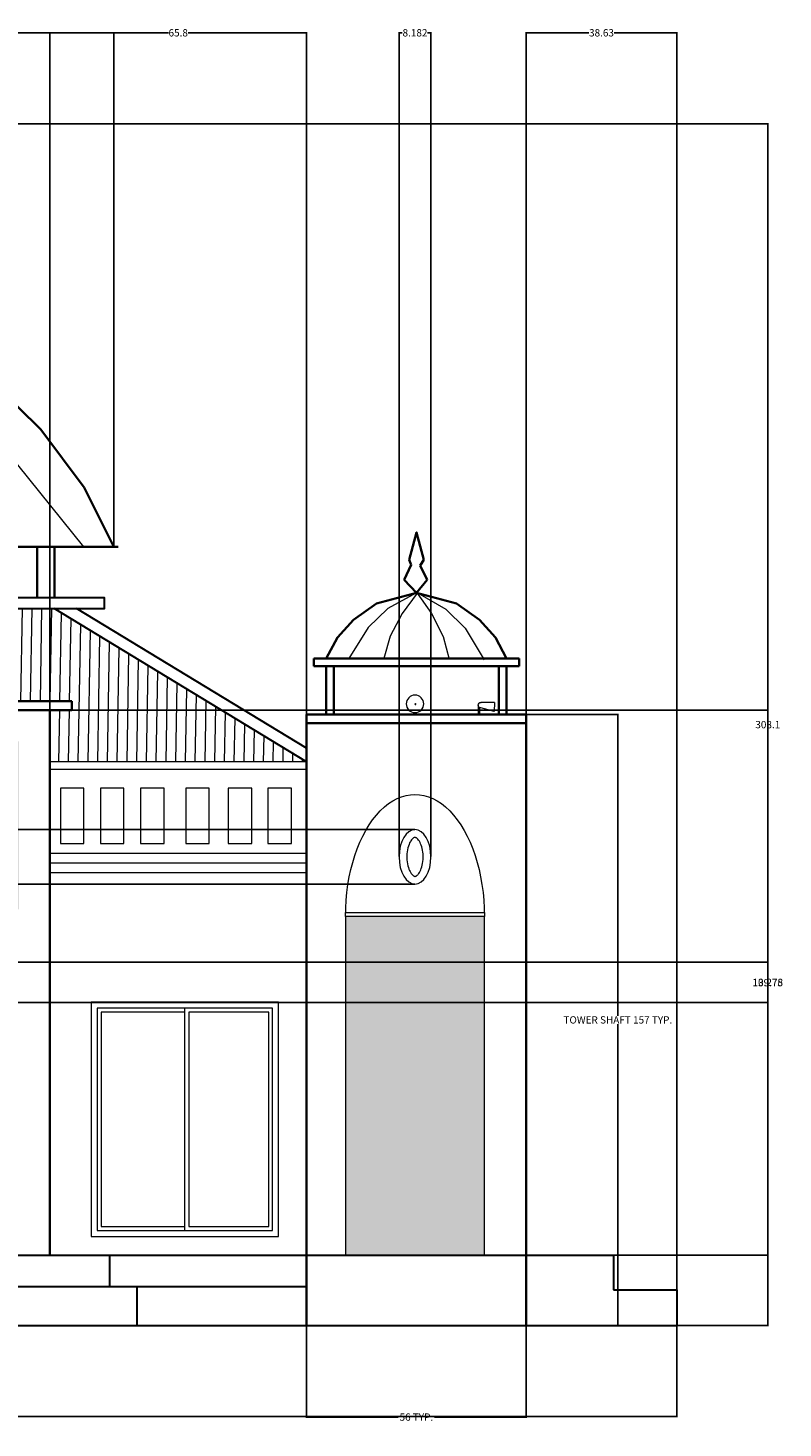
# Model space of a CAD drawing. Units: inches. Extents: x 4 to 523, y 84 to 443.
# Tile 3 of 3: x 329 to 523, y 84 to 443. Entities that reach past the tile are written whole.
import ezdxf

# ---------------------------------------------------------------- set-up
doc = ezdxf.new("R2010")
doc.units = ezdxf.units.IN
doc.header["$MEASUREMENT"] = 0
for name, color, linetype, lineweight in [('A-ANNO-DIMS', 2, 'Continuous', 18), ('A-EQPM', 8, 'Continuous', 18), ('A-FLOR-STRS', 7, 'Continuous', 30), ('A-GLAZ', 4, 'Continuous', 18), ('A-ROOF', 7, 'Continuous', 30), ('A-ROOF-DETL', 3, 'Continuous', 18), ('A-ROOF-DOME', 7, 'Continuous', 35), ('A-ROOF-PATT', 252, 'Continuous', 13), ('A-WALL', 7, 'Continuous', 35), ('A-WALL-PATT', 252, 'Continuous', 13), ('A-WALL-PORT', 7, 'Continuous', 35), ('A-WALL-TRIM', 3, 'Continuous', 18)]:
    doc.layers.add(name, color=color, linetype=linetype, lineweight=lineweight)
doc.styles.get("Standard").update_dxf_attribs({"font": 'arial.ttf'})
doc.dimstyles.get("Standard").update_dxf_attribs({"dimtxt": 1.875, "dimasz": 0.18, "dimexe": 0.18, "dimexo": 0.0625, "dimgap": 0.09, "dimtad": 0, "dimtih": 1, "dimtoh": 1, "dimdec": 4, "dimzin": 0, "dimdsep": 46, "dimlunit": 4, "dimtxsty": 'Standard', "dimcen": 0.09, "dimadec": 0, "dimazin": 0, "dimtfac": 1, "dimtdec": 4, "dimtofl": 0, "dimtmove": 0, "dimatfit": 3, "dimfxl": 1, "dimtolj": 1, "dimtzin": 0, "dimarcsym": 0})

# ---------------------------------------------------------------- blocks, each defined once
blk = doc.blocks.new('*U2')
for p, q in [((1.5, 1.5), (1.5, 58.5)), ((1.5, 58.5), (24, 58.5)), ((24, 1.5), (24, 58.5)), ((24, 58.5), (46.5, 58.5)), ((46.5, 58.5), (46.5, 1.5)), ((24, 1.5), (1.5, 1.5)), ((46.5, 1.5), (24, 1.5))]:
    blk.add_line(p, q)
blk.add_lwpolyline([(0, 0), (0, 60), (48, 60), (48, 0)], close=True)
for points in [[(23, 57.5), (23, 2.5), (2.5, 2.5), (2.5, 57.5), (23, 57.5)], [(24, 57.5), (45.5, 57.5), (45.5, 2.5), (24, 2.5)]]:
    blk.add_lwpolyline(points)
blk = doc.blocks.new('CUPOLA-PROFILE')
for p, q in [((52.59, 14.33), (0, 14.33)), ((0, 14.33), (0, 12.33)), ((0, 12.33), (52.59, 12.33)), ((3.17, 3.77), (3.17, 12.33)), ((5.17, 3.77), (5.17, 12.33)), ((47.49, 3.77), (47.49, 12.33)), ((49.49, 3.77), (49.49, 12.33)), ((52.59, 12.33), (52.59, 14.33)), ((3.17, 3.77), (3.17, 0)), ((5.17, 3.77), (5.17, 0)), ((47.49, 3.77), (47.49, 0)), ((49.49, 3.77), (49.49, 0))]:
    blk.add_line(p, q)
for points in [[(24.44, 39.59), (26.29, 46.64), (28.15, 39.59)], [(25.33, 38.18), (24.44, 39.59)], [(28.15, 39.59), (27.62, 38.34)], [(23.56, 34.47), (25.33, 38.18)], [(29.42, 34.47), (27.62, 38.34)], [(23.56, 34.47), (26.29, 31.2)], [(26.29, 31.2), (29.42, 34.47)], [(3.17, 14.33), (6, 19.75), (10.13, 24.22), (16.05, 28.42), (21.12, 29.8), (26.29, 31.2)], [(49.42, 14.33), (46.59, 19.75), (42.46, 24.22), (36.53, 28.42), (31.46, 29.8), (26.29, 31.2)]]:
    blk.add_lwpolyline(points)
blk = doc.blocks.new('TOWER-LOUDSPEAKERS')
for p, q in [((3.88, 1.79), (3.88, 0)), ((4.17, 2.36), (4.17, 0))]:
    blk.add_line(p, q)
for points in [[(0, 3.08), (0.04, 0.72), (3.47, 1.65)], [(0, 3.08), (3.47, 3.08)]]:
    blk.add_lwpolyline(points)
for centre, radius in [((20.39, 2.69), 2.24), ((20.27, 2.65), 0.127)]:
    blk.add_circle(centre, radius)
blk.add_arc((3.46, 2.36), 0.712, 271.2716, 91.2716)
blk = doc.blocks.new('TOWER-SHAFT')
for p, q in [((0, 0), (0, 156.67)), ((0, 156.67), (56.33, 156.67)), ((0, 154.45), (56.33, 154.45)), ((56.33, 156.67), (56.33, 0))]:
    blk.add_line(p, q)
blk = doc.blocks.new('NICHE-ARCH-MEDALLION')
blk.add_ellipse((17.8, 0), major_axis=(0, 31.26), ratio=0.569254, start_param=4.712389, end_param=7.853982)
blk.add_ellipse((17.8, 15.26), major_axis=(0, 6.99), ratio=0.584915)
blk.add_open_spline([(17.8, 20.25), (17.75, 20.25), (17.71, 20.25), (17.59, 20.21), (17.51, 20.17), (17.31, 20.03), (17.19, 19.93), (16.94, 19.66), (16.81, 19.49), (16.45, 18.9), (16.23, 18.42), (15.9, 17.3), (15.78, 16.67), (15.68, 15.37), (15.7, 14.7), (15.86, 13.43), (16, 12.82), (16.37, 11.77), (16.6, 11.33), (17.01, 10.76), (17.18, 10.58), (17.48, 10.36), (17.59, 10.31), (17.73, 10.26), (17.78, 10.26), (17.87, 10.27), (17.93, 10.28), (18.1, 10.35), (18.21, 10.42), (18.46, 10.64), (18.61, 10.8), (18.9, 11.2), (19.04, 11.44), (19.4, 12.22), (19.6, 12.82), (19.85, 14.13), (19.9, 14.84), (19.86, 16.25), (19.77, 16.94), (19.45, 18.19), (19.23, 18.74), (18.8, 19.48), (18.6, 19.73), (18.25, 20.07), (18.1, 20.16), (17.91, 20.24), (17.85, 20.25), (17.8, 20.25)], degree=3, knots=[0, 0, 0, 0, 0.190161, 0.190161, 0.380322, 0.380322, 0.570483, 0.570483, 0.760644, 0.760644, 1.099719, 1.099719, 1.438794, 1.438794, 1.77787, 1.77787, 2.116945, 2.116945, 2.45602, 2.45602, 2.714331, 2.714331, 2.972641, 2.972641, 3.185337, 3.185337, 3.398033, 3.398033, 3.610729, 3.610729, 3.823425, 3.823425, 4.03612, 4.03612, 4.39902, 4.39902, 4.76192, 4.76192, 5.124819, 5.124819, 5.487719, 5.487719, 5.764017, 5.764017, 6.040315, 6.040315, 6.283185, 6.283185, 6.283185, 6.283185])
blk = doc.blocks.new('FRIEZE-INSET')
blk.add_lwpolyline([(0, 14.2), (6.01, 14.2), (6.01, 0), (0, 0)], close=True)
blk = doc.blocks.new('*D9')
at = {"layer": 'A-ANNO-DIMS', "color": 0, "lineweight": -2, "transparency": 16777216}
for p, q in [((456.93, 267.13), (480.55, 267.13)), ((480.37, 266.95), (480.37, 189.86)), ((480.37, 110.64), (480.37, 187.74)), ((456.93, 110.46), (480.55, 110.46))]:
    blk.add_line(p, q, dxfattribs=at)
at = {"layer": 'A-ANNO-DIMS', "color": 0, "transparency": 16777216}
for points in [[(480.34, 266.95), (480.4, 266.95), (480.37, 267.13)], [(480.34, 110.64), (480.4, 110.64), (480.37, 110.46)]]:
    blk.add_solid(points, dxfattribs=at)
at = {"layer": 'Defpoints', "color": 0, "transparency": 16777216}
for p in [(456.87, 267.13), (480.37, 267.13), (456.87, 110.46)]:
    blk.add_point(p, dxfattribs=at)
at = {"layer": 'A-ANNO-DIMS', "color": 0, "transparency": 16777216, "insert": (480.37, 188.8), "char_height": 1.875, "attachment_point": 5}
blk.add_mtext('\\A1;TOWER SHAFT 157 TYP.', dxfattribs=at)
blk = doc.blocks.new('*D10')
at = {"layer": 'A-ANNO-DIMS', "color": 0, "lineweight": -2, "transparency": 16777216}
for p, q in [((400.53, 110.4), (400.53, 86.78)), ((456.87, 110.4), (456.87, 86.78)), ((400.71, 86.96), (424.05, 86.96)), ((456.69, 86.96), (433.35, 86.96))]:
    blk.add_line(p, q, dxfattribs=at)
at = {"layer": 'A-ANNO-DIMS', "color": 0, "transparency": 16777216}
for points in [[(400.71, 86.99), (400.71, 86.93), (400.53, 86.96)], [(456.69, 86.99), (456.69, 86.93), (456.87, 86.96)]]:
    blk.add_solid(points, dxfattribs=at)
at = {"layer": 'Defpoints', "color": 0, "transparency": 16777216}
for p in [(400.53, 110.46), (456.87, 110.46), (456.87, 86.96)]:
    blk.add_point(p, dxfattribs=at)
at = {"layer": 'A-ANNO-DIMS', "color": 0, "transparency": 16777216, "insert": (428.7, 86.96), "char_height": 1.875, "attachment_point": 5}
blk.add_mtext('\\A1;56 TYP.', dxfattribs=at)
blk = doc.blocks.new('*D19')
at = {"layer": 'A-ANNO-DIMS', "color": 0, "lineweight": -2, "transparency": 16777216}
for p, q in [((30.92, 110.4), (30.92, 86.96)), ((495.5, 110.4), (495.5, 86.96)), ((31.1, 87.14), (259.92, 87.14)), ((495.32, 87.14), (266.5, 87.14))]:
    blk.add_line(p, q, dxfattribs=at)
at = {"layer": 'A-ANNO-DIMS', "color": 0, "transparency": 16777216}
for points in [[(31.1, 87.17), (31.1, 87.11), (30.92, 87.14)], [(495.32, 87.17), (495.32, 87.11), (495.5, 87.14)]]:
    blk.add_solid(points, dxfattribs=at)
at = {"layer": 'Defpoints', "color": 0, "transparency": 16777216}
for p in [(30.92, 110.46), (495.5, 110.46), (495.5, 87.14)]:
    blk.add_point(p, dxfattribs=at)
at = {"layer": 'A-ANNO-DIMS', "color": 0, "transparency": 16777216, "insert": (263.21, 87.14), "char_height": 1.875, "attachment_point": 5}
blk.add_mtext('\\A1;464.6', dxfattribs=at)
blk = doc.blocks.new('*D20')
at = {"layer": 'A-ANNO-DIMS', "color": 0, "lineweight": -2, "transparency": 16777216}
for p, q in [((259.93, 418.56), (519, 418.56)), ((518.82, 418.38), (518.82, 265.56)), ((518.82, 110.64), (518.82, 263.46)), ((495.56, 110.46), (519, 110.46))]:
    blk.add_line(p, q, dxfattribs=at)
at = {"layer": 'A-ANNO-DIMS', "color": 0, "transparency": 16777216}
for points in [[(518.79, 418.38), (518.85, 418.38), (518.82, 418.56)], [(518.79, 110.64), (518.85, 110.64), (518.82, 110.46)]]:
    blk.add_solid(points, dxfattribs=at)
at = {"layer": 'Defpoints', "color": 0, "transparency": 16777216}
for p in [(259.87, 418.56), (518.82, 418.56), (495.5, 110.46)]:
    blk.add_point(p, dxfattribs=at)
at = {"layer": 'A-ANNO-DIMS', "color": 0, "transparency": 16777216, "insert": (518.82, 264.51), "char_height": 1.875, "attachment_point": 5}
blk.add_mtext('\\A1;308.1', dxfattribs=at)
blk = doc.blocks.new('*D22')
at = {"layer": 'A-ANNO-DIMS', "color": 0, "lineweight": -2, "transparency": 16777216}
for p, q in [((456.87, 110.52), (456.87, 442.06)), ((457.05, 441.88), (472.93, 441.88)), ((495.32, 441.88), (479.43, 441.88)), ((495.5, 119.64), (495.5, 442.06))]:
    blk.add_line(p, q, dxfattribs=at)
at = {"layer": 'A-ANNO-DIMS', "color": 0, "transparency": 16777216}
for points in [[(457.05, 441.91), (457.05, 441.85), (456.87, 441.88)], [(495.32, 441.91), (495.32, 441.85), (495.5, 441.88)]]:
    blk.add_solid(points, dxfattribs=at)
at = {"layer": 'Defpoints', "color": 0, "transparency": 16777216}
for p in [(495.5, 441.88), (495.5, 119.58), (456.87, 110.46)]:
    blk.add_point(p, dxfattribs=at)
at = {"layer": 'A-ANNO-DIMS', "color": 0, "transparency": 16777216, "insert": (476.18, 441.88), "char_height": 1.875, "attachment_point": 5}
blk.add_mtext('\\A1;38.63', dxfattribs=at)
blk = doc.blocks.new('*D25')
at = {"layer": 'A-ANNO-DIMS', "color": 0, "lineweight": -2, "transparency": 16777216}
for p, q in [((168.61, 310.13), (168.61, 442.06)), ((168.79, 441.88), (256.7, 441.88)), ((350.95, 441.88), (263.04, 441.88)), ((351.13, 310.13), (351.13, 442.06))]:
    blk.add_line(p, q, dxfattribs=at)
at = {"layer": 'A-ANNO-DIMS', "color": 0, "transparency": 16777216}
for points in [[(168.79, 441.91), (168.79, 441.85), (168.61, 441.88)], [(350.95, 441.91), (350.95, 441.85), (351.13, 441.88)]]:
    blk.add_solid(points, dxfattribs=at)
at = {"layer": 'Defpoints', "color": 0, "transparency": 16777216}
for p in [(351.13, 441.88), (168.61, 310.07), (351.13, 310.07)]:
    blk.add_point(p, dxfattribs=at)
at = {"layer": 'A-ANNO-DIMS', "color": 0, "transparency": 16777216, "insert": (259.87, 441.88), "char_height": 1.875, "attachment_point": 5}
blk.add_mtext('\\A1;182.5', dxfattribs=at)
blk = doc.blocks.new('*D37')
at = {"layer": 'A-ANNO-DIMS', "color": 0, "lineweight": -2, "transparency": 16777216}
for p, q in [((317.98, 203.58), (519, 203.58)), ((518.82, 203.4), (518.82, 199.49)), ((518.82, 193.48), (518.82, 197.4)), ((318.02, 193.3), (519, 193.3))]:
    blk.add_line(p, q, dxfattribs=at)
at = {"layer": 'A-ANNO-DIMS', "color": 0, "transparency": 16777216}
for points in [[(518.79, 203.4), (518.85, 203.4), (518.82, 203.58)], [(518.79, 193.48), (518.85, 193.48), (518.82, 193.3)]]:
    blk.add_solid(points, dxfattribs=at)
at = {"layer": 'Defpoints', "color": 0, "transparency": 16777216}
for p in [(317.92, 203.58), (317.96, 193.3), (518.82, 193.3)]:
    blk.add_point(p, dxfattribs=at)
at = {"layer": 'A-ANNO-DIMS', "color": 0, "transparency": 16777216, "insert": (518.82, 198.44), "char_height": 1.875, "attachment_point": 5}
blk.add_mtext('\\A1;10.278', dxfattribs=at)
blk = doc.blocks.new('*D38')
at = {"layer": 'A-ANNO-DIMS', "color": 0, "lineweight": -2, "transparency": 16777216}
for p, q in [((334.73, 268.28), (334.73, 442.06)), ((334.91, 441.88), (365.1, 441.88)), ((400.35, 441.88), (370.16, 441.88)), ((400.53, 267.19), (400.53, 442.06))]:
    blk.add_line(p, q, dxfattribs=at)
at = {"layer": 'A-ANNO-DIMS', "color": 0, "transparency": 16777216}
for points in [[(334.91, 441.91), (334.91, 441.85), (334.73, 441.88)], [(400.35, 441.91), (400.35, 441.85), (400.53, 441.88)]]:
    blk.add_solid(points, dxfattribs=at)
at = {"layer": 'Defpoints', "color": 0, "transparency": 16777216}
for p in [(400.53, 441.88), (334.73, 268.22), (400.53, 267.13)]:
    blk.add_point(p, dxfattribs=at)
at = {"layer": 'A-ANNO-DIMS', "color": 0, "transparency": 16777216, "insert": (367.63, 441.88), "char_height": 1.875, "attachment_point": 5}
blk.add_mtext('\\A1;65.8', dxfattribs=at)
blk = doc.blocks.new('*D40')
at = {"layer": 'A-ANNO-DIMS', "color": 0, "lineweight": -2, "transparency": 16777216}
for p, q in [((334.79, 268.22), (519, 268.22)), ((518.82, 268.04), (518.82, 199.39)), ((518.82, 128.64), (518.82, 197.29)), ((334.79, 128.46), (519, 128.46))]:
    blk.add_line(p, q, dxfattribs=at)
at = {"layer": 'A-ANNO-DIMS', "color": 0, "transparency": 16777216}
for points in [[(518.79, 268.04), (518.85, 268.04), (518.82, 268.22)], [(518.79, 128.64), (518.85, 128.64), (518.82, 128.46)]]:
    blk.add_solid(points, dxfattribs=at)
at = {"layer": 'Defpoints', "color": 0, "transparency": 16777216}
for p in [(334.73, 268.22), (518.82, 268.22), (334.73, 128.46)]:
    blk.add_point(p, dxfattribs=at)
at = {"layer": 'A-ANNO-DIMS', "color": 0, "transparency": 16777216, "insert": (518.82, 198.34), "char_height": 1.875, "attachment_point": 5}
blk.add_mtext('\\A1;139.75', dxfattribs=at)
blk = doc.blocks.new('*D41')
at = {"layer": 'A-ANNO-DIMS', "color": 0, "lineweight": -2, "transparency": 16777216}
for p, q in [((428.29, 237.59), (7.42, 237.59)), ((7.6, 237.41), (7.6, 231.64)), ((7.6, 223.78), (7.6, 229.55)), ((428.29, 223.6), (7.42, 223.6))]:
    blk.add_line(p, q, dxfattribs=at)
at = {"layer": 'A-ANNO-DIMS', "color": 0, "transparency": 16777216}
for points in [[(7.57, 237.41), (7.63, 237.41), (7.6, 237.59)], [(7.57, 223.78), (7.63, 223.78), (7.6, 223.6)]]:
    blk.add_solid(points, dxfattribs=at)
at = {"layer": 'Defpoints', "color": 0, "transparency": 16777216}
for p in [(428.35, 237.59), (7.6, 223.6), (428.35, 223.6)]:
    blk.add_point(p, dxfattribs=at)
at = {"layer": 'A-ANNO-DIMS', "color": 0, "transparency": 16777216, "insert": (7.6, 230.59), "char_height": 1.875, "attachment_point": 5}
blk.add_mtext('\\A1;13.99', dxfattribs=at)
blk = doc.blocks.new('*D42')
at = {"layer": 'A-ANNO-DIMS', "color": 0, "lineweight": -2, "transparency": 16777216}
for p, q in [((424.26, 230.66), (424.26, 442.06)), ((424.44, 441.88), (425.1, 441.88)), ((432.26, 441.88), (431.59, 441.88)), ((432.44, 230.66), (432.44, 442.06))]:
    blk.add_line(p, q, dxfattribs=at)
at = {"layer": 'A-ANNO-DIMS', "color": 0, "transparency": 16777216}
for points in [[(424.44, 441.91), (424.44, 441.85), (424.26, 441.88)], [(432.26, 441.91), (432.26, 441.85), (432.44, 441.88)]]:
    blk.add_solid(points, dxfattribs=at)
at = {"layer": 'Defpoints', "color": 0, "transparency": 16777216}
for p in [(432.44, 441.88), (424.26, 230.59), (432.44, 230.59)]:
    blk.add_point(p, dxfattribs=at)
at = {"layer": 'A-ANNO-DIMS', "color": 0, "transparency": 16777216, "insert": (428.35, 441.88), "char_height": 1.875, "attachment_point": 5}
blk.add_mtext('\\A1;8.182', dxfattribs=at)

msp = doc.modelspace()

# ---------------------------------------------------------------- hatches: boundary and pattern name
at = {"layer": 'A-ROOF-PATT'}
h = msp.add_hatch(dxfattribs=at)
h.set_pattern_fill('ANSI31', color=256, scale=20, angle=44)
h.paths.add_polyline_path([(335.7846, 294.2465), (329.6848, 294.2465), (259.8699, 294.2465), (190.0549, 294.2465), (183.9551, 294.2465), (119.2078, 254.9874), (185.0083, 254.9874), (185.0083, 259.3969), (185.0083, 268.2159), (179.3813, 268.2159), (179.3813, 270.5155), (240.8614, 270.5155), (259.8699, 270.5155), (278.8783, 270.5155), (340.3584, 270.5155), (340.3584, 268.2159), (334.7314, 268.2159), (334.7314, 259.3969), (334.7314, 254.9874), (400.5319, 254.9874)])
at = {"layer": 'A-WALL-PATT'}
h = msp.add_hatch(dxfattribs=at)
h.set_pattern_fill('ESCHER', color=256, scale=7.5)
h.paths.add_polyline_path([(109.1877, 215.3374), (73.596, 215.3374), (73.596, 128.4611), (109.1877, 128.4611)])
h.paths.add_polyline_path([(446.1437, 215.3374), (410.5521, 215.3374), (410.5521, 128.4611), (446.1437, 128.4611)])
h.paths.add_polyline_path([(326.7314, 260.2159), (259.8699, 260.2159), (193.0083, 260.2159), (193.0083, 217.1172), (203.3352, 217.1172), (207.1721, 217.1172, -0.58399271), (312.6778, 217.1172), (316.4045, 217.1172), (326.7314, 217.1172)])

# ---------------------------------------------------------------- linework, layer by layer
at = {"layer": 'A-FLOR-STRS'}
for p, q in [((62.873, 128.4611), (463.5437, 128.4611)), ((349.9956, 128.4611), (349.9956, 120.483)), ((463.5437, 128.4611), (479.2655, 128.4611)), ((479.2655, 128.4611), (479.2655, 119.5803)), ((119.2078, 120.483), (400.5319, 120.483)), ((357.0414, 120.483), (357.0414, 110.4611)), ((479.2655, 119.5803), (495.4954, 119.5803)), ((495.4954, 119.5803), (495.4954, 110.4611)), ((229.6366, 110.4611), (465.7812, 110.4611)), ((465.7812, 110.4611), (495.4954, 110.4611))]:
    msp.add_line(p, q, dxfattribs=at)
at = {"layer": 'A-ROOF'}
for p, q in [((400.5319, 254.9874), (335.7846, 294.2465)), ((400.5319, 258.4958), (341.5707, 294.2465))]:
    msp.add_line(p, q, dxfattribs=at)
msp.add_lwpolyline([(259.8699, 294.2465), (329.6848, 294.2465), (348.7111, 294.2465), (348.7111, 296.9786), (259.8699, 296.9786)], dxfattribs=at)
at = {"layer": 'A-ROOF-DETL'}
for points in [[(262.3558, 380.5683), (283.1606, 370.8672), (306.2195, 356.0749), (343.3375, 310.0699)], [(428.7311, 298.3291), (421.4226, 294.2762), (416.3719, 289.4369), (411.3903, 281.4574)], [(428.8788, 298.1745), (425.0896, 293.0318), (421.9761, 287.2246), (420.3156, 281.4574)], [(428.8788, 298.1745), (432.5766, 292.9656), (435.5869, 287.1044), (437.1453, 281.3087)], [(429.0293, 298.3264), (436.265, 294.145), (441.2294, 289.2172), (446.0691, 281.1509)]]:
    msp.add_lwpolyline(points, dxfattribs=at)
at = {"layer": 'A-ROOF-DOME'}
for p, q in [((352.2366, 310.0699), (294.5837, 310.0699)), ((331.4715, 301.3423), (331.4715, 310.0699)), ((335.8733, 301.3423), (335.8733, 310.0699)), ((331.4715, 301.3423), (331.4715, 296.9786)), ((335.8733, 301.3423), (335.8733, 296.9786))]:
    msp.add_line(p, q, dxfattribs=at)
msp.add_lwpolyline([(351.128, 310.0699), (343.5316, 325.3117), (332.4318, 340.1657), (314.791, 357.3962), (298.5377, 368.091), (280.6987, 376.4092), (264.8418, 380.5683), (259.8699, 380.5683)], dxfattribs=at)
at = {"layer": 'A-WALL-PORT'}
for p, q in [((340.3584, 270.5155), (278.8783, 270.5155)), ((340.3584, 270.5155), (340.3584, 268.2159)), ((334.7314, 268.2159), (259.8699, 268.2159)), ((334.7314, 259.3969), (334.7314, 268.2159)), ((334.7314, 268.2159), (340.3584, 268.2159)), ((334.7314, 259.3969), (334.7314, 254.9874)), ((334.7314, 254.9874), (334.7314, 128.4611))]:
    msp.add_line(p, q, dxfattribs=at)
at = {"layer": 'A-WALL-TRIM'}
for p, q in [((400.5319, 254.9874), (334.7314, 254.9874)), ((400.5319, 252.9874), (334.7314, 252.9874)), ((400.5319, 231.4916), (334.7314, 231.4916)), ((400.5319, 228.9916), (334.7314, 228.9916)), ((400.5319, 226.4916), (334.7314, 226.4916)), ((410.5617, 216.3641), (446.1346, 216.3365))]:
    msp.add_line(p, q, dxfattribs=at)
msp.add_lwpolyline([(446.1437, 215.3374), (410.5521, 215.3374), (410.5521, 128.4611), (446.1437, 128.4611)], close=True, dxfattribs=at)

# ---------------------------------------------------------------- block references
at = {"layer": 'A-EQPM', "extrusion": (0, 0, -1), "zscale": -1}
msp.add_blockref('TOWER-LOUDSPEAKERS', (-448.7317, 267.131), dxfattribs=at)
at = {"layer": 'A-GLAZ', "xscale": -1, "rotation": 359.9999999999999}
msp.add_blockref('*U2', (393.3301, 133.3038), dxfattribs=at)
at = {"layer": 'A-ROOF-DOME', "extrusion": (0, 0, -1), "zscale": -1}
msp.add_blockref('CUPOLA-PROFILE', (-455.0257, 267.131), dxfattribs=at)
at = {"layer": 'A-WALL'}
msp.add_blockref('TOWER-SHAFT', (400.5319, 110.461), dxfattribs=at)
at = {"layer": 'A-WALL-TRIM', "extrusion": (0, 0, -1), "zscale": -1}
for name, p in [('FRIEZE-INSET', (-343.4403, 234.017)), ('FRIEZE-INSET', (-353.674, 234.017)), ('FRIEZE-INSET', (-363.9891, 234.017)), ('FRIEZE-INSET', (-375.6036, 234.017)), ('FRIEZE-INSET', (-386.4871, 234.017)), ('FRIEZE-INSET', (-396.6397, 234.017)), ('NICHE-ARCH-MEDALLION', (-446.1437, 215.337))]:
    msp.add_blockref(name, p, dxfattribs=at)

# ---------------------------------------------------------------- dimensions: what is measured, and where the dimension line sits
at = {"layer": 'A-ANNO-DIMS'}
for base, p1, p2, override, picture, middle in [((351.128, 441.8826), (168.6117, 310.0699), (351.128, 310.0699), {"dimdec": 1, "dimlfac": 1, "dimrnd": 0, "dimzin": 0, "dimdsep": 46, "dimlunit": 2}, '*D25', (259.8699, 441.8826)), ((400.5319, 441.8826), (334.7314, 268.2159), (400.5319, 267.1306), {"dimdec": 1, "dimlfac": 1, "dimrnd": 0, "dimzin": 0, "dimdsep": 46, "dimlunit": 2}, '*D38', (367.6317, 441.8826)), ((432.439, 441.8826), (424.2567, 230.595), (432.439, 230.595), {"dimdec": 3, "dimlfac": 1, "dimrnd": 0, "dimzin": 0, "dimdsep": 46, "dimlunit": 2}, '*D42', (428.3479, 441.8826)), ((495.4954, 441.8826), (456.8667, 110.4611), (495.4954, 119.5803), {"dimdec": 2, "dimlfac": 1, "dimrnd": 0, "dimzin": 0, "dimdsep": 46, "dimlunit": 2}, '*D22', (476.181, 441.8826)), ((495.4954, 87.1361), (30.9213, 110.4611), (495.4954, 110.4611), {"dimdec": 1, "dimlfac": 1, "dimrnd": 0, "dimzin": 0, "dimdsep": 46, "dimlunit": 2}, '*D19', (263.2083, 87.1361))]:
    dim = msp.add_linear_dim(base=base, p1=p1, p2=p2, dimstyle='Standard', override=override, dxfattribs=at)
    dim.commit()
    dim.dimension.update_dxf_attribs({"geometry": picture, "text_midpoint": middle})
for base, p1, p2, override, picture, middle in [((518.8204, 418.5576), (495.4954, 110.4611), (259.8702, 418.5576), {"dimdec": 1, "dimlfac": 1, "dimrnd": 0, "dimzin": 0, "dimdsep": 46, "dimlunit": 2}, '*D20', (518.8204, 264.5094)), ((518.8204, 268.2159), (334.7314, 128.4611), (334.7314, 268.2159), {"dimdec": 2, "dimlfac": 1, "dimrnd": 0, "dimzin": 0, "dimdsep": 46, "dimlunit": 2}, '*D40', (518.8204, 198.3385)), ((7.5963, 223.6005), (428.3479, 237.5894), (428.3479, 223.6005), {"dimdec": 2, "dimlfac": 1, "dimrnd": 0, "dimzin": 0, "dimdsep": 46, "dimlunit": 2}, '*D41', (7.5963, 230.595)), ((518.8204, 193.3038), (317.9162, 203.5817), (317.9616, 193.3038), {"dimdec": 3, "dimlfac": 1, "dimrnd": 0, "dimzin": 0, "dimdsep": 46, "dimlunit": 2}, '*D37', (518.8204, 198.4427))]:
    dim = msp.add_linear_dim(base=base, p1=p1, p2=p2, angle=90, dimstyle='Standard', override=override, dxfattribs=at)
    dim.commit()
    dim.dimension.update_dxf_attribs({"geometry": picture, "text_midpoint": middle})
dim = msp.add_linear_dim(base=(480.3671, 267.1306), p1=(456.8667, 110.4611), p2=(456.8667, 267.1306), angle=90, text='TOWER SHAFT <> TYP.', dimstyle='Standard', override={"dimdec": 0, "dimlfac": 1, "dimrnd": 0, "dimzin": 0, "dimdsep": 46, "dimlunit": 2}, dxfattribs=at)
dim.commit()
dim.dimension.update_dxf_attribs({"geometry": '*D9', "text_midpoint": (480.3671, 188.7958)})
dim = msp.add_linear_dim(base=(456.8667, 86.9606), p1=(400.5319, 110.4611), p2=(456.8667, 110.4611), text='<> TYP.', dimstyle='Standard', override={"dimdec": 0, "dimlfac": 1, "dimrnd": 0, "dimzin": 0, "dimdsep": 46, "dimlunit": 2}, dxfattribs=at)
dim.commit()
dim.dimension.update_dxf_attribs({"geometry": '*D10', "text_midpoint": (428.6993, 86.9606)})

doc.saveas('drawing.dxf')
